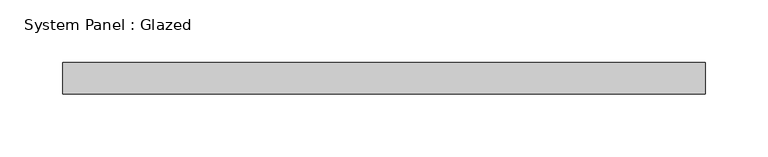
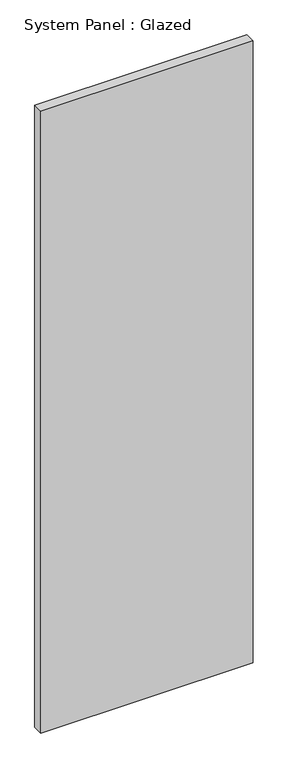
"""IFC4 building model written with IfcOpenShell, lengths in millimetres: plate geometry, System Panel : Glazed."""

from ifc_helpers import new_model, si_unit, origin, origin_with_axes, place, context, project, spatial, polyline, outline, extrude, source, transform, mapped, element, save


def system_panel_glazed_080605c3(model_context):
    return source(origin(), model_context, "Body", "SweptSolid", [
        extrude(outline(polyline([(257.175, 19.05), (-257.175, 19.05), (-257.175, 44.45), (257.175, 44.45), (257.175, 19.05)])), origin_with_axes(), (0.0, 0.0, 1.0), 1593.7849865),
    ])


if __name__ == "__main__":
    model = new_model("IFC4")
    model_context = context("Model", 3, world=origin())
    ifc_project = project(units=[si_unit("LENGTHUNIT", "METRE", prefix="MILLI")], contexts=[model_context])
    site = spatial("IfcSite", under=ifc_project)
    building = spatial("IfcBuilding", under=site)
    placement = place(None, origin())
    system_panel_glazed_shape = system_panel_glazed_080605c3(model_context)
    element("IfcPlate", 1, ObjectType="System Panel : Glazed", at=placement, inside=building, context=model_context, shape_type="MappedRepresentation", body=[
        mapped(system_panel_glazed_shape, transform((0.0, 0.0, 0.0), x_axis=(1.0, 0.0, 0.0), y_axis=(0.0, 1.0, 0.0), z_axis=(0.0, 0.0, 1.0))),
    ])
    save(model, "model.ifc")

# Revit data of these elements
# Type "System Panel : Glazed"
#   Construction Type Id = "GSP4R"
#   Analytic Construction = "1/8 in Pilkington single glazing"
#   Visual Light Transmittance = 0.9
#   Solar Heat Gain Coefficient = 0.86
#   Heat Transfer Coefficient (U) = 1.18115 BTU/(h·ft²·°F)
#   Define Thermal Properties by = 1
# Element 1 (IfcPlate, "System Panel : Glazed")
#   Materials on its faces: "Glass"
# Materials
#   "Glass": class "Glass", colour RGB 0 128 192, transparency 0.75, Description = "Soda Lime Glass", Cost = 0
